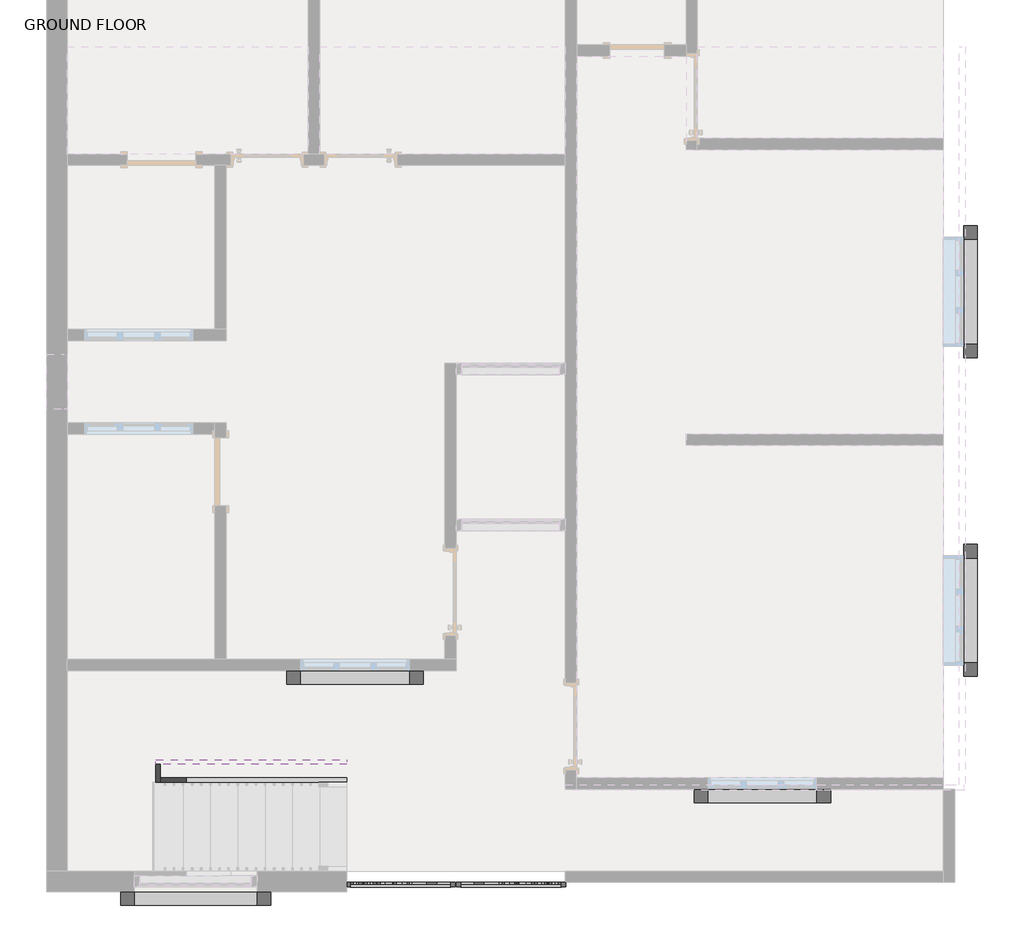
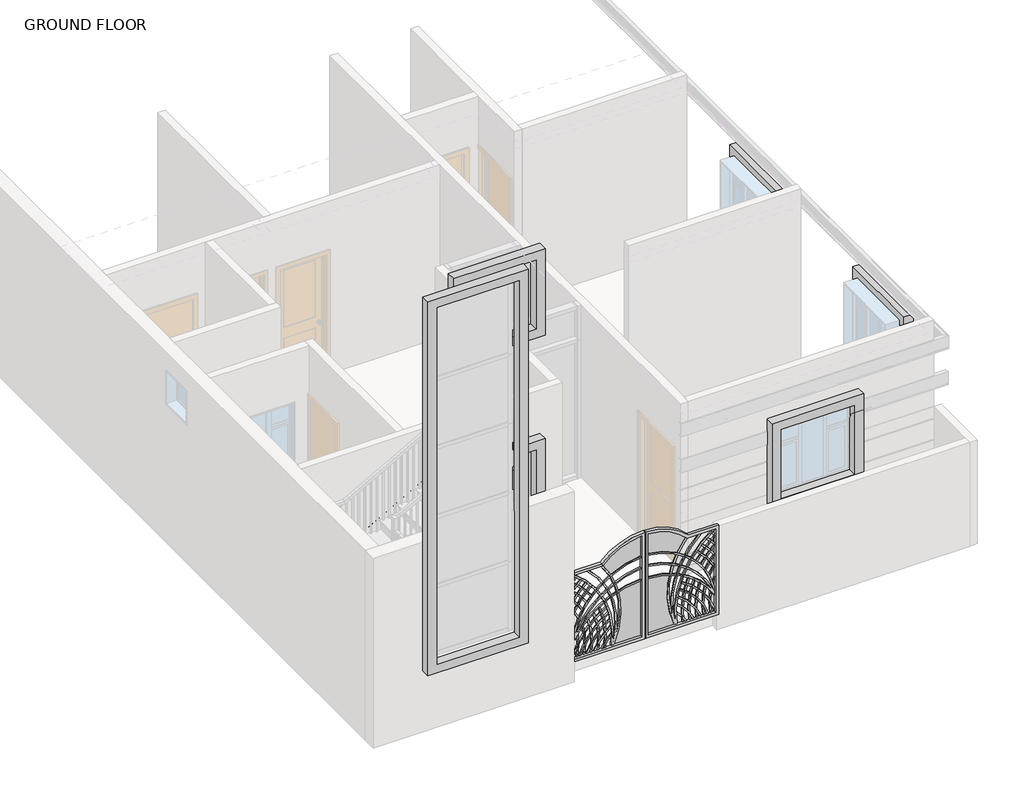
# One storey, part 7 of 7: 6 proxies, 4 members.
"""IFC4 building model written with IfcOpenShell, lengths in millimetres."""

from ifc_helpers import new_model, si_unit, frame, origin, place, context, project, spatial, polyline, outline, extrude, transform, mapped, element, save
from components import generic_models_6bc30956, generic_models_2_generic_models_2_a6d57641, generic_models_4_generic_models_4_fb6d851a, generic_models_3_generic_models_3_0ad4c425, generic_models_6_generic_models_6_ceaf88ca

model = new_model("IFC4")

# Units and contexts
model_context = context("Model", 3, world=origin())
ifc_project = project(units=[si_unit("LENGTHUNIT", "METRE", prefix="MILLI")], contexts=[model_context])

# Site, building, storey
site = spatial("IfcSite", under=ifc_project)
building = spatial("IfcBuilding", under=site)
storey = spatial("IfcBuildingStorey", under=building, Name="GROUND FLOOR", Elevation=304.8)

# Proxies
placement = place(None, origin())
generic_models_shape = generic_models_6bc30956(model_context)
element("IfcBuildingElementProxy", 1, Name="Generic Models", at=placement, inside=storey, context=model_context, shape_type="MappedRepresentation", body=[
    mapped(generic_models_shape, transform((-10430.0023867, -2883.7499863, 304.8), x_axis=(1.0, 0.0, 0.0), y_axis=(0.0, 1.0, 0.0), z_axis=(0.0, 0.0, 1.0))),
])
generic_models_2_generic_models_2_shape = generic_models_2_generic_models_2_a6d57641(model_context)
element("IfcBuildingElementProxy", 2, Name="Generic Models 2 : Generic Models 2", ObjectType="Generic Models 2 : Generic Models 2", at=placement, inside=storey, context=model_context, shape_type="MappedRepresentation", body=[
    mapped(generic_models_2_generic_models_2_shape, transform((0.0, 0.0, 0.0), x_axis=(1.0, 0.0, 0.0), y_axis=(0.0, 1.0, 0.0), z_axis=(0.0, 0.0, 1.0))),
])
generic_models_4_generic_models_4_shape = generic_models_4_generic_models_4_fb6d851a(model_context)
element("IfcBuildingElementProxy", 3, Name="Generic Models 4 : Generic Models 4", ObjectType="Generic Models 4 : Generic Models 4", at=placement, inside=storey, context=model_context, shape_type="MappedRepresentation", body=[
    mapped(generic_models_4_generic_models_4_shape, transform((0.0, 0.0, 0.0), x_axis=(1.0, 0.0, 0.0), y_axis=(0.0, 1.0, 0.0), z_axis=(0.0, 0.0, 1.0))),
])
generic_models_3_generic_models_3_shape = generic_models_3_generic_models_3_0ad4c425(model_context)
element("IfcBuildingElementProxy", 4, Name="Generic Models 5 : Generic Models 3", ObjectType="Generic Models 5 : Generic Models 3", at=placement, inside=storey, context=model_context, shape_type="MappedRepresentation", body=[
    mapped(generic_models_3_generic_models_3_shape, transform((0.0, 0.0, -3352.8), x_axis=(1.0, 0.0, 0.0), y_axis=(0.0, 1.0, 0.0), z_axis=(0.0, 0.0, 1.0))),
])
generic_models_6_generic_models_6_shape = generic_models_6_generic_models_6_ceaf88ca(model_context)
element("IfcBuildingElementProxy", 5, Name="Generic Models 8 : Generic Models 6", ObjectType="Generic Models 8 : Generic Models 6", at=placement, inside=storey, context=model_context, shape_type="MappedRepresentation", body=[
    mapped(generic_models_6_generic_models_6_shape, transform((0.0, 3556.0, -3362.9203125), x_axis=(1.0, 0.0, 0.0), y_axis=(0.0, 1.0, 0.0), z_axis=(0.0, 0.0, 1.0))),
])
element("IfcBuildingElementProxy", 6, Name="Generic Models 9 : Generic Models 6", ObjectType="Generic Models 9 : Generic Models 6", at=placement, inside=storey, context=model_context, shape_type="MappedRepresentation", body=[
    mapped(generic_models_6_generic_models_6_shape, transform((0.0, 0.0, -3352.8), x_axis=(1.0, 0.0, 0.0), y_axis=(0.0, 1.0, 0.0), z_axis=(0.0, 0.0, 1.0))),
])

# Members
element("IfcMember", 7, ObjectType="Stringer - 2\" Width", at=placement, inside=storey, context=model_context, shape_type="SweptSolid", body=[
    extrude(outline(polyline([(1430.8666667, -13927.6378839), (2703.7197207, -11636.5023867), (3052.3983948, -11636.5023867), (1430.8666667, -14555.2594973), (1430.8666667, -13927.6378839)])), frame((0.0, -521.5499863, 0.0), z_axis=(0.0, 1.0, 0.0), x_axis=(0.0, 0.0, 1.0)), (0.0, 0.0, 1.0), 50.8),
])
element("IfcMember", 8, ObjectType="Stringer - 2\" Width", at=placement, inside=storey, context=model_context, shape_type="SweptSolid", body=[
    extrude(outline(polyline([(304.8, -11636.5023867), (512.3983948, -11636.5023867), (1669.5095059, -13719.3023867), (1320.8308318, -13719.3023867), (304.8, -11890.4468895), (304.8, -11636.5023867)])), frame((0.0, -1766.1499863, 0.0), z_axis=(0.0, 1.0, 0.0), x_axis=(0.0, 0.0, 1.0)), (0.0, 0.0, 1.0), 50.8),
])
element("IfcMember", 9, ObjectType="Stringer - 2\" Width", at=placement, inside=storey, context=model_context, shape_type="SweptSolid", body=[
    extrude(outline(polyline([(-13719.3023867, -1766.1499863), (-13770.1023867, -1766.1499863), (-13770.1023867, -1562.9499863), (-13719.3023867, -1562.9499863), (-13719.3023867, -1766.1499863)])), frame((0.0, 0.0, 1430.8666667), z_axis=(0.0, 0.0, 1.0), x_axis=(1.0, 0.0, 0.0)), (0.0, 0.0, 1.0), 304.8),
])
element("IfcMember", 10, ObjectType="Stringer - 2\" Width", at=placement, inside=storey, context=model_context, shape_type="SweptSolid", body=[
    extrude(outline(polyline([(1867.0650614, -13770.1023867), (1518.3863873, -13770.1023867), (2703.7197207, -11636.5023867), (3052.3983948, -11636.5023867), (1867.0650614, -13770.1023867)])), frame((0.0, -1562.9499863, 0.0), z_axis=(0.0, 1.0, 0.0), x_axis=(0.0, 0.0, 1.0)), (0.0, 0.0, 1.0), 50.8),
])

save(model, "model.ifc")

# Revit data of these elements
# Type
#   m.s. sheet = none
#   2" x2" pipe = none
#   1"x1"pipe = none
#   Default Elevation = 0
# Element 1 (IfcBuildingElementProxy)
#   Phase Created = New Construction
# Element 2 (IfcBuildingElementProxy, "Generic Models 2 : Generic Models 2")
#   Phase Created = New Construction
#   Materials on its faces: "accent wall"
# Element 3 (IfcBuildingElementProxy, "Generic Models 4 : Generic Models 4")
#   Phase Created = New Construction
#   Materials on its faces: "accent wall"
# Element 4 (IfcBuildingElementProxy, "Generic Models 5 : Generic Models 3")
#   Phase Created = New Construction
#   Materials on its faces: "accent wall"
# Element 5 (IfcBuildingElementProxy, "Generic Models 8 : Generic Models 6")
#   Phase Created = New Construction
#   Materials on its faces: "accent wall"
# Element 6 (IfcBuildingElementProxy, "Generic Models 9 : Generic Models 6")
#   Phase Created = New Construction
#   Materials on its faces: "accent wall"
# Elements 7, 8, 9, 10 (IfcMember, "Stringer - 2\" Width")
#   Phase Created = New Construction
# Materials
#   "accent wall": class "Generic", colour RGB 120 120 120, transparency 0, Cost = 0
